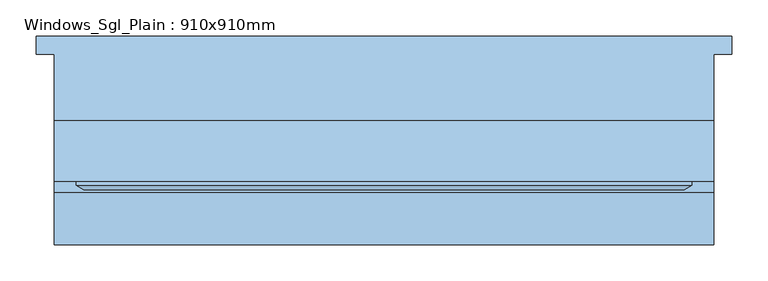
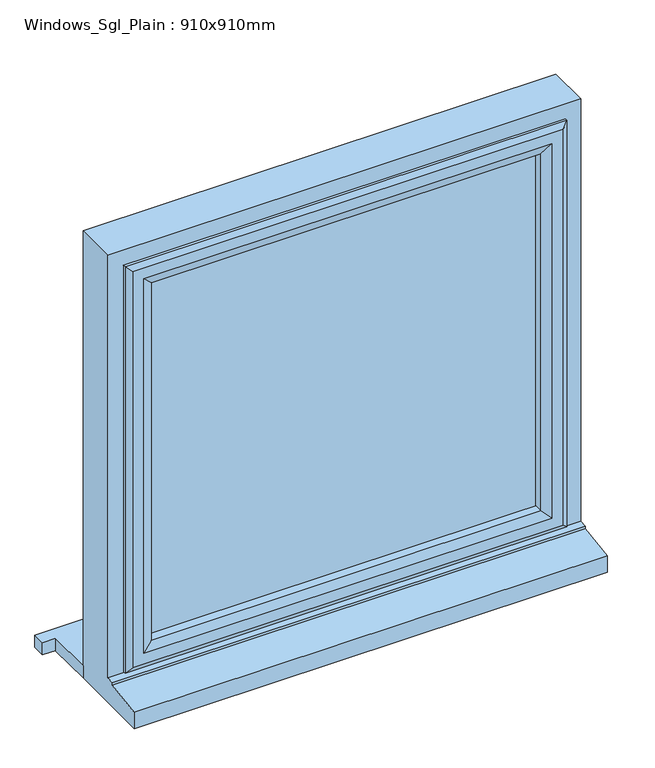
"""IFC4 building model written with IfcOpenShell, lengths in millimetres: window geometry, Windows_Sgl_Plain : 910x910mm."""

from ifc_helpers import new_model, si_unit, frame, origin, place, context, project, spatial, polyline, outline, extrude, faceted_brep, source, transform, mapped, element, save


def windows_sgl_plain_910x910mm_23580505(model_context):
    return source(origin(), model_context, "Body", "SolidModel", [
        extrude(outline(polyline([(-480.0, 129.0434322), (480.0, 129.0434322), (480.0, 104.0434322), (455.0, 104.0434322), (455.0, 12.0434322), (-455.0, 12.0434322), (-455.0, 104.0434322), (-480.0, 104.0434322), (-480.0, 129.0434322)])), frame((0.0, 0.0, 1200.0), z_axis=(0.0, 0.0, 1.0), x_axis=(1.0, 0.0, 0.0)), (0.0, 0.0, 1.0), 25.0),
        faceted_brep([(-455.0, 12.0434322, 1200.0), (-455.0, 12.0434322, 2110.0), (455.0, 12.0434322, 2110.0), (455.0, 12.0434322, 1200.0), (-395.0, 12.0434322, 2050.0), (-395.0, 12.0434322, 1275.0), (395.0, 12.0434322, 1275.0), (395.0, 12.0434322, 2050.0), (-455.0, -158.4565678, 1200.0), (-455.0, -158.4565678, 1233.8088847), (-455.0, -85.9565678, 1244.7449676), (-455.0, -85.9565678, 1249.68767), (-455.0, -70.9565678, 1251.0), (-455.0, -70.9565678, 2110.0), (455.0, -70.9565678, 1251.0), (455.0, -70.9565678, 2110.0), (-415.0, -70.9565678, 2070.0), (415.0, -70.9565678, 2070.0), (415.0, -70.9565678, 1263.0), (-415.0, -70.9565678, 1263.0), (-415.0, -5.9565678, 1263.0), (-415.0, -5.9565678, 2070.0), (415.0, -5.9565678, 1263.0), (415.0, -5.9565678, 2070.0), (-395.0, -5.9565678, 2050.0), (395.0, -5.9565678, 2050.0), (395.0, -5.9565678, 1275.0), (-395.0, -5.9565678, 1275.0), (455.0, -85.9565678, 1249.68767), (455.0, -85.9565678, 1244.7449676), (455.0, -158.4565678, 1233.8088847), (455.0, -158.4565678, 1200.0)], [[[0, 1, 2, 3], [4, 5, 6, 7]], [[0, 8, 9, 10, 11, 12, 13, 1]], [[12, 14, 15, 13], [16, 17, 18, 19]], [[19, 20, 21, 16]], [[21, 20, 22, 23], [24, 25, 26, 27]], [[24, 27, 5, 4]], [[1, 13, 15, 2]], [[16, 21, 23, 17]], [[7, 25, 24, 4]], [[14, 28, 29, 30, 31, 3, 2, 15]], [[17, 23, 22, 18]], [[7, 6, 26, 25]], [[31, 8, 0, 3]], [[30, 9, 8, 31]], [[29, 10, 9, 30]], [[28, 11, 10, 29]], [[14, 12, 11, 28]], [[20, 19, 18, 22]], [[5, 27, 26, 6]]]),
        extrude(outline(polyline([(385.0, -34.9565678), (385.0, -58.9565678), (-385.0, -58.9565678), (-385.0, -34.9565678), (385.0, -34.9565678)])), frame((0.0, 0.0, 1293.0), z_axis=(0.0, 0.0, 1.0), x_axis=(1.0, 0.0, 0.0)), (0.0, 0.0, 1.0), 747.0),
        faceted_brep([(-425.0, -70.9565678, 2080.0), (-425.0, -70.9565678, 1253.0), (-425.0, -76.7300705, 1253.0), (-425.0, -76.7300705, 2080.0), (-415.0, -5.9565678, 2070.0), (-415.0, -5.9565678, 1263.0), (-415.0, -70.9565678, 1263.0), (-415.0, -70.9565678, 2070.0), (-375.0, -20.4494677, 2030.0), (-375.0, -20.4494677, 1303.0), (-385.1480377, -5.9565678, 1292.8519623), (-385.1480377, -5.9565678, 2040.1480377), (-375.0, -34.9565678, 2030.0), (-375.0, -34.9565678, 1303.0), (-385.0, -58.9565678, 2040.0), (-385.0, -58.9565678, 1293.0), (-385.0, -34.9565678, 1293.0), (-385.0, -34.9565678, 2040.0), (-375.0, -76.7300705, 2030.0), (-375.0, -76.7300705, 1303.0), (-375.0, -58.9565678, 1303.0), (-375.0, -58.9565678, 2030.0), (-392.4457548, -82.5035732, 2047.4457548), (-392.4457548, -82.5035732, 1285.5542452), (-414.2153903, -82.5035732, 1263.7846097), (-414.2153903, -82.5035732, 2069.2153903), (425.0, -70.9565678, 1253.0), (425.0, -76.7300705, 1253.0), (415.0, -5.9565678, 1263.0), (415.0, -70.9565678, 1263.0), (375.0, -20.4494677, 1303.0), (385.1480377, -5.9565678, 1292.8519623), (375.0, -34.9565678, 1303.0), (385.0, -58.9565678, 1293.0), (385.0, -34.9565678, 1293.0), (375.0, -76.7300705, 1303.0), (375.0, -58.9565678, 1303.0), (392.4457548, -82.5035732, 1285.5542452), (414.2153903, -82.5035732, 1263.7846097), (425.0, -70.9565678, 2080.0), (425.0, -76.7300705, 2080.0), (415.0, -5.9565678, 2070.0), (415.0, -70.9565678, 2070.0), (375.0, -20.4494677, 2030.0), (385.1480377, -5.9565678, 2040.1480377), (375.0, -34.9565678, 2030.0), (385.0, -58.9565678, 2040.0), (385.0, -34.9565678, 2040.0), (375.0, -76.7300705, 2030.0), (375.0, -58.9565678, 2030.0), (392.4457548, -82.5035732, 2047.4457548), (414.2153903, -82.5035732, 2069.2153903)], [[[0, 1, 2, 3]], [[4, 5, 6, 7]], [[8, 9, 10, 11]], [[12, 13, 9, 8]], [[14, 15, 16, 17]], [[18, 19, 20, 21]], [[22, 23, 19, 18]], [[3, 2, 24, 25]], [[1, 26, 27, 2]], [[5, 28, 29, 6]], [[9, 30, 31, 10]], [[13, 32, 30, 9]], [[15, 33, 34, 16]], [[19, 35, 36, 20]], [[23, 37, 35, 19]], [[2, 27, 38, 24]], [[26, 39, 40, 27]], [[28, 41, 42, 29]], [[30, 43, 44, 31]], [[32, 45, 43, 30]], [[33, 46, 47, 34]], [[35, 48, 49, 36]], [[37, 50, 48, 35]], [[27, 40, 51, 38]], [[39, 0, 3, 40]], [[1, 0, 39, 26], [7, 6, 29, 42]], [[41, 4, 7, 42]], [[5, 4, 41, 28], [11, 10, 31, 44]], [[43, 8, 11, 44]], [[45, 12, 8, 43]], [[17, 16, 34, 47], [13, 12, 45, 32]], [[46, 14, 17, 47]], [[15, 14, 46, 33], [21, 20, 36, 49]], [[48, 18, 21, 49]], [[50, 22, 18, 48]], [[25, 24, 38, 51], [23, 22, 50, 37]], [[40, 3, 25, 51]]]),
    ])


if __name__ == "__main__":
    model = new_model("IFC4")
    model_context = context("Model", 3, world=origin())
    ifc_project = project(units=[si_unit("LENGTHUNIT", "METRE", prefix="MILLI")], contexts=[model_context])
    site = spatial("IfcSite", under=ifc_project)
    building = spatial("IfcBuilding", under=site)
    placement = place(None, origin())
    windows_sgl_plain_910x910mm_shape = windows_sgl_plain_910x910mm_23580505(model_context)
    element("IfcWindow", 1, ObjectType="Windows_Sgl_Plain : 910x910mm", at=placement, inside=building, context=model_context, shape_type="MappedRepresentation", body=[
        mapped(windows_sgl_plain_910x910mm_shape, transform((0.0, 0.0, 0.0), x_axis=(1.0, 0.0, 0.0), y_axis=(0.0, 1.0, 0.0), z_axis=(0.0, 0.0, 1.0))),
    ])
    save(model, "model.ifc")

# Revit data of these elements
# Type "Windows_Sgl_Plain : 910x910mm"
#   Type Mark = "44"
#   Operation = "SinglePanel"
#   Construction Type Id = "SGL"
#   Manufacturer = "Revit"
#   Keynote = "L10"
#   Analytic Construction = "Large single-glazed windows"
#   Wrap Layers (Ext) from Ext = 102.5 mm
#   Wrap Layers (Int) from Ext = 177.5 mm
#   Window Board Projection = 25 mm
#   Window Board Extension = 25 mm
#   Visual Light Transmittance = 0.9
#   Solar Heat Gain Coefficient = 0.86
#   Rough Width = 910 mm
#   Rough Height = 910 mm
#   Height = 910 mm
#   Width = 910 mm
#   Heat Transfer Coefficient (U) = 5.5617 W/(m²·K)
#   Glazing Thickness = 24 mm
#   FrameOffset - External = 50 mm
#   Frame Depth = 65 mm
#   Default Head Height = 2110 mm
#   Cill Depth = 87.5 mm
#   Cavity Closer Width = 50 mm
#   Cavity Closer Offset from Ext = 102.5 mm
#   Cavity Closer Depth = 85 mm
#   Define Thermal Properties by = 1
#   Vis - Cavity Closers = yes
#   Define Thermal Properties by = 1
#   Material Trim = Window Frame
#   Material Glass = Glass
#   Material Frame = Window Frame
#   Wall Closure = (empty or 0)
# Element 1 (IfcWindow, "Windows_Sgl_Plain : 910x910mm")
#   Materials on its faces: "Window Frame", "Glass"
# Materials
#   "Window Frame": colour RGB 249 249 249, transparency 0, Keynote = "L10", Cost = 0
#   "Glass": class "Glass", colour RGB 0 128 192, transparency 0.9, Description = "Soda Lime Glass", Cost = 0
